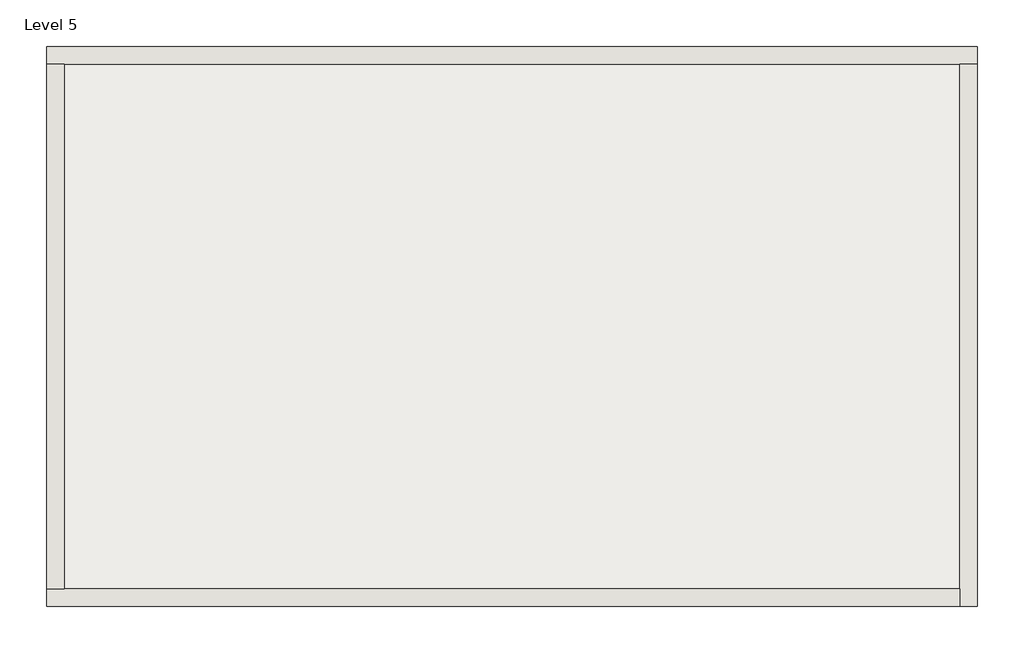
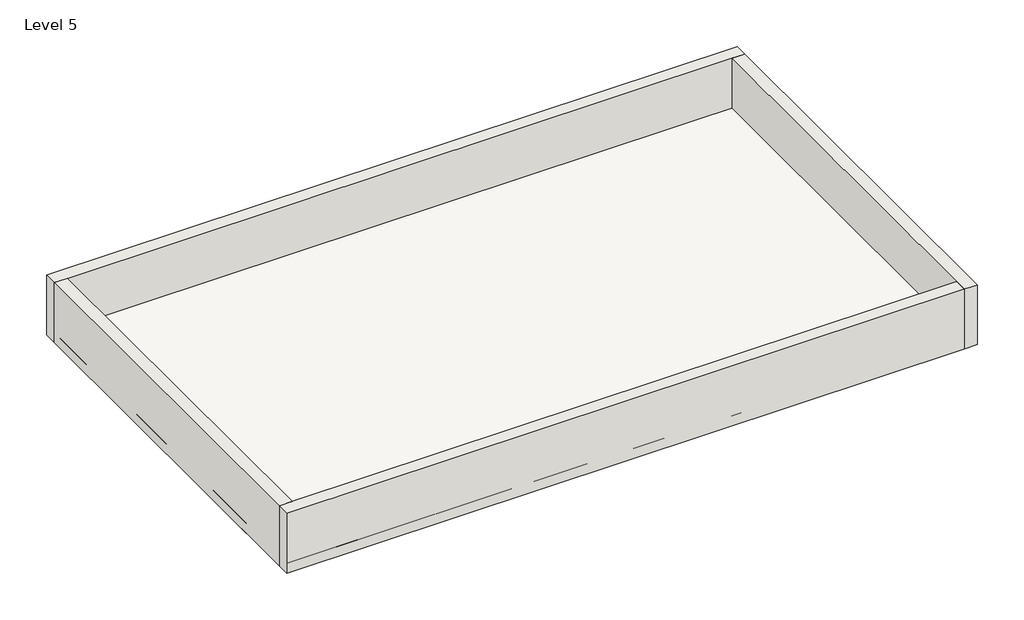
# One storey: 4 walls, 1 roof.
"""IFC4 building model written with IfcOpenShell, lengths in millimetres."""

from ifc_helpers import new_model, si_unit, frame, origin, place, context, project, spatial, polyline, outline, extrude, faceted_brep, element, save

model = new_model("IFC4")

# Units and contexts
model_context = context("Model", 3, world=origin())
ifc_project = project(units=[si_unit("LENGTHUNIT", "METRE", prefix="MILLI")], contexts=[model_context])

# Site, building, storey
site = spatial("IfcSite", under=ifc_project)
building = spatial("IfcBuilding", under=site)
storey = spatial("IfcBuildingStorey", under=building, Name="Level 5", Elevation=12192.0)

# Roof
placement = place(None, origin())
element("IfcRoof", 1, ObjectType="Generic - 4\"", at=placement, inside=storey, context=model_context, shape_type="SweptSolid", body=[
    extrude(outline(polyline([(-2910.36646, -604.5834702), (3757.13354, -604.5834702), (3757.13354, -4617.7834702), (-2910.36646, -4617.7834702), (-2910.36646, -604.5834702)])), frame((0.0, 0.0, 12192.0), z_axis=(0.0, 0.0, 1.0), x_axis=(1.0, 0.0, 0.0)), (0.0, 0.0, 1.0), 101.6),
])

# Walls
element("IfcWall", 2, ObjectType="Generic - 5\"", at=placement, inside=storey, context=model_context, shape_type="Brep", body=[
    faceted_brep([(-2910.36646, -731.5834702, 12192.0), (-2783.36646, -731.5834702, 12192.0), (3630.13354, -731.5834702, 12192.0), (3757.13354, -731.5834702, 12192.0), (3757.13354, -731.5834702, 12801.6), (3630.13354, -731.5834702, 12801.6), (-2783.36646, -731.5834702, 12801.6), (-2910.36646, -731.5834702, 12801.6), (-2910.36646, -604.5834702, 12192.0), (-2910.36646, -604.5834702, 12801.6), (3757.13354, -604.5834702, 12801.6), (3757.13354, -604.5834702, 12192.0)], [[[0, 1, 2, 3, 4, 5, 6, 7]], [[8, 9, 10, 11]], [[3, 2, 1, 0, 8, 11]], [[7, 6, 5, 4, 10, 9]], [[4, 3, 11, 10]], [[0, 7, 9, 8]]]),
])
element("IfcWall", 3, ObjectType="Generic - 5\"", at=placement, inside=storey, context=model_context, shape_type="Brep", body=[
    faceted_brep([(3630.13354, -731.5834702, 12192.0), (3630.13354, -4490.7834702, 12192.0), (3630.13354, -4617.7834702, 12192.0), (3630.13354, -4617.7834702, 12801.6), (3630.13354, -4490.7834702, 12801.6), (3630.13354, -731.5834702, 12801.6), (3757.13354, -731.5834702, 12192.0), (3757.13354, -731.5834702, 12801.6), (3757.13354, -4617.7834702, 12801.6), (3757.13354, -4617.7834702, 12192.0)], [[[0, 1, 2, 3, 4, 5]], [[6, 7, 8, 9]], [[2, 1, 0, 6, 9]], [[5, 4, 3, 8, 7]], [[0, 5, 7, 6]], [[3, 2, 9, 8]]]),
])
element("IfcWall", 4, ObjectType="Generic - 5\"", at=placement, inside=storey, context=model_context, shape_type="Brep", body=[
    faceted_brep([(3630.13354, -4490.7834702, 12192.0), (-2783.36646, -4490.7834702, 12192.0), (-2910.36646, -4490.7834702, 12192.0), (-2910.36646, -4490.7834702, 12801.6), (-2783.36646, -4490.7834702, 12801.6), (3630.13354, -4490.7834702, 12801.6), (3630.13354, -4617.7834702, 12192.0), (3630.13354, -4617.7834702, 12801.6), (-2910.36646, -4617.7834702, 12801.6), (-2910.36646, -4617.7834702, 12192.0)], [[[0, 1, 2, 3, 4, 5]], [[6, 7, 8, 9]], [[2, 1, 0, 6, 9]], [[5, 4, 3, 8, 7]], [[0, 5, 7, 6]], [[3, 2, 9, 8]]]),
])
element("IfcWall", 5, ObjectType="Generic - 5\"", at=placement, inside=storey, context=model_context, shape_type="SweptSolid", body=[
    extrude(outline(polyline([(-2783.36646, -731.5834702), (-2783.36646, -4490.7834702), (-2910.36646, -4490.7834702), (-2910.36646, -731.5834702), (-2783.36646, -731.5834702)])), frame((0.0, 0.0, 12192.0), z_axis=(0.0, 0.0, 1.0), x_axis=(1.0, 0.0, 0.0)), (0.0, 0.0, 1.0), 609.6),
])

save(model, "model.ifc")

# Revit data of these elements
# Type "Generic - 4\""
#   Assembly Code = "B1020"
#   Layers, outside or top first: 0' - 4" no material (function 1)
# Type "Generic - 5\""
#   Assembly Code = "B2010"
#   Layers, outside or top first: 0' - 5" no material (function 1)
# Element 1 (IfcRoof, "Generic - 4\"")
#   built-in parameter 1001705 = 40.3333 (stored number, unit not read)
#   built-in parameter 1001710 = 33615
#   Phase Created = New Construction
#   Materials on its faces: "Default Roof"
# Elements 2, 5 (IfcWall, "Generic - 5\"")
#   Top Offset = 0' - 0"
#   Base Offset = 0' - 0"
#   Unconnected Height = 2' - 0"
#   wall height = 2' - 0"
#   Phase Created = New Construction
#   Base Constraint = Level 5
#   Materials on its faces: "Default Wall"
# Elements 3, 4 (IfcWall, "Generic - 5\"")
#   Top Offset = 0' - 0"
#   Base Offset = 0' - 0"
#   Unconnected Height = 2' - 0"
#   wall height = 2' - 0"
#   Phase Created = New Construction
#   Base Constraint = Level 5
#   Materials on its faces: "Default Wall", "01 colour"
# Materials
#   "Default Roof": colour RGB 80 80 80, transparency 0
#   "Default Wall": colour RGB 80 80 80, transparency 0
#   "01 colour": class "Generic", colour RGB 120 120 120, transparency 0, Cost = 0
